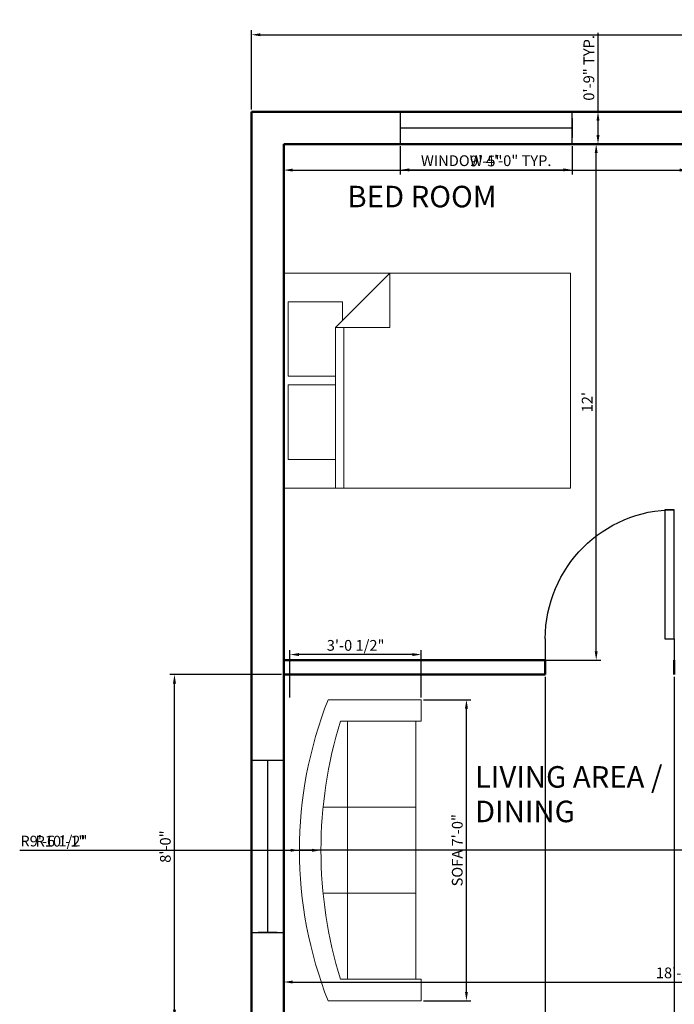
# Model space of a CAD drawing. Units: inches. Extents: x 1767 to 2185, y 3382 to 3854.
# Tile 2 of 4: x 1767 to 1950, y 3577 to 3852. Entities that reach past the tile are written whole.
import ezdxf

# ---------------------------------------------------------------- set-up
doc = ezdxf.new("R2010")
doc.units = ezdxf.units.IN
for name, color, linetype, lineweight in [('A-ANNO-DIMS', 2, 'Continuous', 18), ('A-AREA-IDEN', 7, 'Continuous', 25), ('A-DOOR', 3, 'Continuous', 25), ('A-FURN', 8, 'Continuous', 18), ('A-GLAZ', 4, 'Continuous', 25), ('A-WALL', 7, 'Continuous', 50)]:
    doc.layers.add(name, color=color, linetype=linetype, lineweight=lineweight)
doc.styles.get("Standard").update_dxf_attribs({"font": 'arial.ttf'})
doc.dimstyles.new('ISO-25', dxfattribs={"dimtxt": 3, "dimasz": 2.5, "dimexe": 1.25, "dimexo": 0.625, "dimtad": 1, "dimdec": 0, "dimlunit": 3, "dimtxsty": 'Standard', "dimcen": 2.5, "dimadec": 0, "dimazin": 0, "dimtfac": 1, "dimtdec": 0, "dimtmove": 0, "dimatfit": 3, "dimfxl": 1, "dimarcsym": 0})

# ---------------------------------------------------------------- blocks, each defined once
blk = doc.blocks.new('*U2')
for p, q in [((0, 0), (0, -100)), ((600, 0), (600, -100))]:
    blk.add_line(p, q)
blk.add_lwpolyline([(0, 0), (0, 600), (43.75, 600), (43.75, 0)], close=True)
blk.add_arc((0, 0), 600, 0, 90)
blk = doc.blocks.new('*U4')
for p, q in [((0, 100), (0, 0)), ((900, 100), (900, 0)), ((0, 50), (900, 50))]:
    blk.add_line(p, q)
blk = doc.blocks.new('Bed - Queen')
for p, q in [((0, -80.00003), (0, 0)), ((0, 0), (59.99999, 0)), ((59.99999, 0), (59.99999, -80.00003)), ((7.99999, -1.2), (28.79998, -1.2)), ((7.99999, -14.4), (7.99999, -1.2)), ((28.79998, -1.2), (28.79998, -14.4)), ((31.19999, -1.2), (51.99999, -1.2)), ((31.19999, -14.4), (31.19999, -1.2)), ((51.99999, -1.2), (51.99999, -16.4)), ((0, -14.4), (44.8, -14.4)), ((59.99999, -29.6), (44.8, -14.4)), ((44.8, -14.4), (44.8, -29.6)), ((51.99999, -16.4), (46.79936, -16.4)), ((44.8, -16.8), (0, -16.8)), ((44.8, -29.6), (59.99999, -29.6)), ((59.99999, -80.00003), (0, -80.00003))]:
    blk.add_line(p, q)
blk = doc.blocks.new('Sofa - Roundback 7 ft.')
for p, q in [((-12.00002, -32.4421), (-12.00003, -6.5971)), ((11.99997, -32.4421), (11.99998, -6.5971)), ((-36.000027, -34), (-36.000027, -11.4696)), ((-35.999844, -13.3819), (35.9998, -13.3819)), ((35.99998, -34), (35.99998, -11.4696)), ((-36.000027, -32.4421), (35.99998, -32.4421))]:
    blk.add_line(p, q)
for points in [[(-36.000027, -34), (-42.000027, -34), (-42.000027, -8)], [(41.99998, -8), (41.99998, -34), (35.99998, -34)]]:
    blk.add_lwpolyline(points)
for centre, radius, start, end in [((0, -114.25), 114.25, 68.43141, 111.5686), ((-0.00001, -127.1968), 121.1968, 72.72033, 107.2797)]:
    blk.add_arc(centre, radius, start, end)
blk = doc.blocks.new('*D10')
at = {"layer": 'A-ANNO-DIMS', "color": 0, "lineweight": -2, "transparency": 16777216}
for p, q in [((1841.16, 3816.53), (1841.16, 3808.64)), ((1954.16, 3816.53), (1954.16, 3808.64)), ((1843.66, 3809.89), (1951.66, 3809.89))]:
    blk.add_line(p, q, dxfattribs=at)
at = {"layer": 'A-ANNO-DIMS', "color": 0, "transparency": 16777216}
for points in [[(1843.66, 3810.31), (1843.66, 3809.48), (1841.16, 3809.89)], [(1951.66, 3810.31), (1951.66, 3809.48), (1954.16, 3809.89)]]:
    blk.add_solid(points, dxfattribs=at)
at = {"layer": 'Defpoints', "color": 0, "transparency": 16777216}
for p in [(1841.16, 3817.15), (1954.16, 3817.15), (1954.16, 3809.89)]:
    blk.add_point(p, dxfattribs=at)
at = {"layer": 'A-ANNO-DIMS', "color": 0, "transparency": 16777216, "insert": (1897.66, 3812.05), "char_height": 3, "attachment_point": 5}
blk.add_mtext('9\'-5"', dxfattribs=at)
blk = doc.blocks.new('*D11')
at = {"layer": 'A-ANNO-DIMS', "color": 0, "lineweight": -2, "transparency": 16777216}
for p, q in [((1841.78, 3817.15), (1929.61, 3817.15)), ((1928.36, 3675.65), (1928.36, 3814.65)), ((1841.78, 3673.15), (1929.61, 3673.15))]:
    blk.add_line(p, q, dxfattribs=at)
at = {"layer": 'A-ANNO-DIMS', "color": 0, "transparency": 16777216}
for points in [[(1927.94, 3814.65), (1928.77, 3814.65), (1928.36, 3817.15)], [(1927.94, 3675.65), (1928.77, 3675.65), (1928.36, 3673.15)]]:
    blk.add_solid(points, dxfattribs=at)
at = {"layer": 'Defpoints', "color": 0, "transparency": 16777216}
for p in [(1841.16, 3817.15), (1928.36, 3817.15), (1841.16, 3673.15)]:
    blk.add_point(p, dxfattribs=at)
at = {"layer": 'A-ANNO-DIMS', "color": 0, "transparency": 16777216, "insert": (1926.23, 3745.15), "char_height": 3, "attachment_point": 5, "rotation": 90}
blk.add_mtext("12'", dxfattribs=at)
blk = doc.blocks.new('*D17')
at = {"layer": 'A-ANNO-DIMS', "color": 0, "lineweight": -2, "transparency": 16777216}
for p, q in [((1841.16, 3668.53), (1841.16, 3582.12)), ((2060.16, 3668.53), (2060.16, 3582.12)), ((1843.66, 3583.37), (2057.66, 3583.37))]:
    blk.add_line(p, q, dxfattribs=at)
at = {"layer": 'A-ANNO-DIMS', "color": 0, "transparency": 16777216}
for points in [[(1843.66, 3583.79), (1843.66, 3582.96), (1841.16, 3583.37)], [(2057.66, 3583.79), (2057.66, 3582.96), (2060.16, 3583.37)]]:
    blk.add_solid(points, dxfattribs=at)
at = {"layer": 'Defpoints', "color": 0, "transparency": 16777216}
for p in [(1841.16, 3669.15), (2060.16, 3669.15), (2060.16, 3583.37)]:
    blk.add_point(p, dxfattribs=at)
at = {"layer": 'A-ANNO-DIMS', "color": 0, "transparency": 16777216, "insert": (1950.66, 3585.53), "char_height": 3, "attachment_point": 5}
blk.add_mtext('18\'-3"', dxfattribs=at)
blk = doc.blocks.new('WIN-OPENING-48IN-WALL-9IN')
for p, q in [((48, 9), (0, 9)), ((0, 9), (0, 0)), ((48, 0), (48, 9))]:
    blk.add_line(p, q)
blk = doc.blocks.new('*D27')
at = {"layer": 'A-ANNO-DIMS', "color": 0, "lineweight": -2, "transparency": 16777216}
for p, q in [((1873.66, 3816.53), (1873.66, 3808.7)), ((1921.66, 3816.53), (1921.66, 3808.7)), ((1876.16, 3809.95), (1919.16, 3809.95))]:
    blk.add_line(p, q, dxfattribs=at)
at = {"layer": 'A-ANNO-DIMS', "color": 0, "transparency": 16777216}
for points in [[(1876.16, 3810.37), (1876.16, 3809.53), (1873.66, 3809.95)], [(1919.16, 3810.37), (1919.16, 3809.53), (1921.66, 3809.95)]]:
    blk.add_solid(points, dxfattribs=at)
at = {"layer": 'Defpoints', "color": 0, "transparency": 16777216}
for p in [(1873.66, 3817.15), (1921.66, 3817.15), (1921.66, 3809.95)]:
    blk.add_point(p, dxfattribs=at)
at = {"layer": 'A-ANNO-DIMS', "color": 0, "transparency": 16777216, "insert": (1897.66, 3812.13), "char_height": 3, "attachment_point": 5}
blk.add_mtext('WINDOW 4\'-0" TYP.', dxfattribs=at)
blk = doc.blocks.new('*D28')
at = {"layer": 'A-ANNO-DIMS', "color": 0, "lineweight": -2, "transparency": 16777216}
for p, q in [((1928.86, 3826.15), (1928.86, 3848.19)), ((1922.28, 3826.15), (1930.11, 3826.15)), ((1928.86, 3819.65), (1928.86, 3823.65)), ((1922.28, 3817.15), (1930.11, 3817.15))]:
    blk.add_line(p, q, dxfattribs=at)
at = {"layer": 'A-ANNO-DIMS', "color": 0, "transparency": 16777216}
for points in [[(1928.44, 3823.65), (1929.28, 3823.65), (1928.86, 3826.15)], [(1928.44, 3819.65), (1929.28, 3819.65), (1928.86, 3817.15)]]:
    blk.add_solid(points, dxfattribs=at)
at = {"layer": 'Defpoints', "color": 0, "transparency": 16777216}
for p in [(1921.66, 3826.15), (1928.86, 3826.15), (1921.66, 3817.15)]:
    blk.add_point(p, dxfattribs=at)
at = {"layer": 'A-ANNO-DIMS', "color": 0, "transparency": 16777216, "insert": (1926.7, 3838.42), "char_height": 3, "attachment_point": 5, "rotation": 90}
blk.add_mtext('0\'-9" TYP.', dxfattribs=at)
blk = doc.blocks.new('*D37')
at = {"layer": 'A-ANNO-DIMS', "color": 0, "lineweight": -2, "transparency": 16777216}
for p, q in [((1880.17, 3662.13), (1893.39, 3662.13)), ((1892.14, 3580.63), (1892.14, 3659.63)), ((1880.17, 3578.13), (1893.39, 3578.13))]:
    blk.add_line(p, q, dxfattribs=at)
at = {"layer": 'A-ANNO-DIMS', "color": 0, "transparency": 16777216}
for points in [[(1891.73, 3659.63), (1892.56, 3659.63), (1892.14, 3662.13)], [(1891.73, 3580.63), (1892.56, 3580.63), (1892.14, 3578.13)]]:
    blk.add_solid(points, dxfattribs=at)
at = {"layer": 'Defpoints', "color": 0, "transparency": 16777216}
for p in [(1879.54, 3662.13), (1892.14, 3662.13), (1879.54, 3578.13)]:
    blk.add_point(p, dxfattribs=at)
at = {"layer": 'A-ANNO-DIMS', "color": 0, "transparency": 16777216, "insert": (1889.97, 3620.13), "char_height": 3, "attachment_point": 5, "rotation": 90}
blk.add_mtext('SOFA 7\'-0"', dxfattribs=at)
blk = doc.blocks.new('*D38')
at = {"layer": 'A-ANNO-DIMS', "color": 0, "lineweight": -2, "transparency": 16777216}
for p, q in [((1842.88, 3662.75), (1842.88, 3675.98)), ((1879.54, 3662.75), (1879.54, 3675.98)), ((1877.04, 3674.73), (1845.38, 3674.73))]:
    blk.add_line(p, q, dxfattribs=at)
at = {"layer": 'A-ANNO-DIMS', "color": 0, "transparency": 16777216}
for points in [[(1845.38, 3675.14), (1845.38, 3674.31), (1842.88, 3674.73)], [(1877.04, 3675.14), (1877.04, 3674.31), (1879.54, 3674.73)]]:
    blk.add_solid(points, dxfattribs=at)
at = {"layer": 'Defpoints', "color": 0, "transparency": 16777216}
for p in [(1842.88, 3674.73), (1842.88, 3662.13), (1879.54, 3662.13)]:
    blk.add_point(p, dxfattribs=at)
at = {"layer": 'A-ANNO-DIMS', "color": 0, "transparency": 16777216, "insert": (1861.21, 3676.9), "char_height": 3, "attachment_point": 5}
blk.add_mtext('3\'-0 1/2"', dxfattribs=at)
blk = doc.blocks.new('*D39')
at = {"layer": 'A-ANNO-DIMS', "color": 0, "lineweight": -2, "transparency": 16777216}
for p, q in [((1832.16, 3826.78), (1832.16, 3848.91)), ((2144.16, 3826.78), (2144.16, 3848.91)), ((1834.66, 3847.66), (2141.66, 3847.66))]:
    blk.add_line(p, q, dxfattribs=at)
at = {"layer": 'A-ANNO-DIMS', "color": 0, "transparency": 16777216}
for points in [[(1834.66, 3848.07), (1834.66, 3847.24), (1832.16, 3847.66)], [(2141.66, 3848.07), (2141.66, 3847.24), (2144.16, 3847.66)]]:
    blk.add_solid(points, dxfattribs=at)
at = {"layer": 'Defpoints', "color": 0, "transparency": 16777216}
for p in [(2144.16, 3847.66), (1832.16, 3826.15), (2144.16, 3826.15)]:
    blk.add_point(p, dxfattribs=at)
at = {"layer": 'A-ANNO-DIMS', "color": 0, "transparency": 16777216, "insert": (1988.16, 3849.81), "char_height": 3, "attachment_point": 5}
blk.add_mtext('26\'-0"', dxfattribs=at)
blk = doc.blocks.new('*D41')
at = {"layer": 'A-ANNO-DIMS', "color": 0, "lineweight": -2, "transparency": 16777216}
for p, q in [((1840.53, 3669.15), (1809.4, 3669.15)), ((1810.65, 3575.65), (1810.65, 3666.65)), ((1831.53, 3573.15), (1809.4, 3573.15))]:
    blk.add_line(p, q, dxfattribs=at)
at = {"layer": 'A-ANNO-DIMS', "color": 0, "transparency": 16777216}
for points in [[(1810.24, 3666.65), (1811.07, 3666.65), (1810.65, 3669.15)], [(1810.24, 3575.65), (1811.07, 3575.65), (1810.65, 3573.15)]]:
    blk.add_solid(points, dxfattribs=at)
at = {"layer": 'Defpoints', "color": 0, "transparency": 16777216}
for p in [(1810.65, 3669.15), (1841.16, 3669.15), (1832.16, 3573.15)]:
    blk.add_point(p, dxfattribs=at)
at = {"layer": 'A-ANNO-DIMS', "color": 0, "transparency": 16777216, "insert": (1808.5, 3621.15), "char_height": 3, "attachment_point": 5, "rotation": 90}
blk.add_mtext('8\'-0"', dxfattribs=at)
blk = doc.blocks.new('*D42')
at = {"layer": 'A-ANNO-DIMS', "color": 0, "lineweight": -2, "transparency": 16777216}
for p, q in [((1914.16, 3668.53), (1914.16, 3383.4)), ((1950.16, 3668.53), (1950.16, 3383.4)), ((1916.66, 3384.65), (1947.66, 3384.65))]:
    blk.add_line(p, q, dxfattribs=at)
at = {"layer": 'A-ANNO-DIMS', "color": 0, "transparency": 16777216}
for points in [[(1916.66, 3385.06), (1916.66, 3384.23), (1914.16, 3384.65)], [(1947.66, 3385.06), (1947.66, 3384.23), (1950.16, 3384.65)]]:
    blk.add_solid(points, dxfattribs=at)
at = {"layer": 'Defpoints', "color": 0, "transparency": 16777216}
for p in [(1914.16, 3669.15), (1950.16, 3669.15), (1950.16, 3384.65)]:
    blk.add_point(p, dxfattribs=at)
at = {"layer": 'A-ANNO-DIMS', "color": 0, "transparency": 16777216, "insert": (1932.16, 3386.8), "char_height": 3, "attachment_point": 5}
blk.add_mtext('3\'-0"', dxfattribs=at)
blk = doc.blocks.new('*D51')
at = {"layer": 'A-ANNO-DIMS', "color": 0, "lineweight": -2, "transparency": 16777216}
for p, q in [((1771.61, 3620.13), (1849.04, 3620.13)), ((1972.74, 3620.13), (1851.54, 3620.13))]:
    blk.add_line(p, q, dxfattribs=at)
at = {"layer": 'A-ANNO-DIMS', "color": 0, "transparency": 16777216}
blk.add_solid([(1849.04, 3620.54), (1849.04, 3619.71), (1851.54, 3620.13)], dxfattribs=at)
at = {"layer": 'Defpoints', "color": 0, "transparency": 16777216}
for p in [(1851.54, 3620.13), (1972.74, 3620.13)]:
    blk.add_point(p, dxfattribs=at)
at = {"layer": 'A-ANNO-DIMS', "color": 0, "transparency": 16777216, "insert": (1778.83, 3622.28), "char_height": 3, "attachment_point": 5, "rotation": 359.9999}
blk.add_mtext('R10\'-1"', dxfattribs=at)
blk = doc.blocks.new('*D52')
at = {"layer": 'A-ANNO-DIMS', "color": 0, "lineweight": -2, "transparency": 16777216}
for p, q in [((1767.45, 3620.13), (1843.04, 3620.13)), ((1959.79, 3620.13), (1845.54, 3620.13))]:
    blk.add_line(p, q, dxfattribs=at)
at = {"layer": 'A-ANNO-DIMS', "color": 0, "transparency": 16777216}
blk.add_solid([(1843.04, 3620.54), (1843.04, 3619.71), (1845.54, 3620.13)], dxfattribs=at)
at = {"layer": 'Defpoints', "color": 0, "transparency": 16777216}
for p in [(1845.54, 3620.13), (1959.79, 3620.13)]:
    blk.add_point(p, dxfattribs=at)
at = {"layer": 'A-ANNO-DIMS', "color": 0, "transparency": 16777216, "insert": (1776.99, 3622.3), "char_height": 3, "attachment_point": 5, "rotation": 359.9999}
blk.add_mtext('R9\'-6 1/2"', dxfattribs=at)

msp = doc.modelspace()

# ---------------------------------------------------------------- linework, layer by layer
at = {"layer": 'A-WALL'}
for p, q in [((1832.16, 3826.15), (2144.16, 3826.15)), ((1832.16, 3406.15), (1832.16, 3826.15)), ((1841.16, 3415.15), (1841.16, 3817.15)), ((1841.16, 3817.15), (2135.16, 3817.15)), ((1841.16, 3673.15), (1914.16, 3673.15)), ((1914.16, 3673.15), (1914.16, 3669.15)), ((1950.16, 3669.15), (1950.16, 3673.15)), ((1841.16, 3669.15), (1914.16, 3669.15))]:
    msp.add_line(p, q, dxfattribs=at)

# ---------------------------------------------------------------- block references
at = {"layer": 'A-DOOR', "xscale": -0.0599999999999998, "yscale": 0.0599999999999998, "zscale": 0.0599999999999998}
msp.add_blockref('*U2', (1950.16, 3679.15), dxfattribs=at)
at = {"layer": 'A-FURN', "rotation": 90}
for name, p in [('Bed - Queen', (1841.16, 3721.16)), ('Sofa - Roundback 7 ft.', (1845.54, 3620.13))]:
    msp.add_blockref(name, p, dxfattribs=at)
at = {"layer": 'A-GLAZ'}
msp.add_blockref('WIN-OPENING-48IN-WALL-9IN', (1873.66, 3817.15), dxfattribs=at)
at = {"layer": 'A-GLAZ', "xscale": 0.0533333333333335, "yscale": 0.0533333333333335, "zscale": 0.0533333333333335}
msp.add_blockref('*U4', (1873.66, 3818.98), dxfattribs=at)
at = {"layer": 'A-GLAZ', "rotation": 90.00000000000126}
msp.add_blockref('WIN-OPENING-48IN-WALL-9IN', (1841.16, 3597.15), dxfattribs=at)
at = {"layer": 'A-GLAZ', "xscale": 0.0533333333333335, "yscale": 0.0533333333333335, "zscale": 0.0533333333333335, "rotation": 270}
msp.add_blockref('*U4', (1833.99, 3645.15), dxfattribs=at)

# ---------------------------------------------------------------- texts
at = {"layer": 'A-AREA-IDEN'}
for s, p in [('BED ROOM', (1858.91, 3799.51)), ('LIVING AREA /', (1894.5, 3637.6)), ('DINING', (1894.5, 3627.96))]:
    msp.add_text(s, height=6, dxfattribs=at).set_placement(p)

# ---------------------------------------------------------------- dimensions: what is measured, and where the dimension line sits
at = {"layer": 'A-ANNO-DIMS'}
for base, p1, p2, override, picture, middle in [((2144.16, 3847.66), (1832.16, 3826.15), (2144.16, 3826.15), {"dimdec": 1, "dimlfac": 1, "dimrnd": 0, "dimzin": 1, "dimdsep": 46, "dimlunit": 4, "dimfrac": 2}, '*D39', (1988.16, 3849.81)), ((1954.16, 3809.89), (1841.16, 3817.15), (1954.16, 3817.15), {"dimclrd": 0, "dimclre": 0, "dimclrt": 0}, '*D10', (1897.66, 3812.05)), ((2060.16, 3583.37), (1841.16, 3669.15), (2060.16, 3669.15), {"dimclrd": 0, "dimclre": 0, "dimclrt": 0}, '*D17', (1950.66, 3585.53)), ((1950.16, 3384.65), (1914.16, 3669.15), (1950.16, 3669.15), {"dimdec": 1, "dimlfac": 1, "dimrnd": 0, "dimzin": 1, "dimdsep": 46, "dimlunit": 4, "dimfrac": 2}, '*D42', (1932.16, 3386.8))]:
    dim = msp.add_linear_dim(base=base, p1=p1, p2=p2, dimstyle='ISO-25', override=override, dxfattribs=at)
    dim.commit()
    dim.dimension.update_dxf_attribs({"geometry": picture, "text_midpoint": middle})
for base, p1, p2, text, picture, middle in [((1928.86, 3826.15), (1921.66, 3817.15), (1921.66, 3826.15), '<> TYP.', '*D28', (1926.7, 3838.42)), ((1892.14, 3662.13), (1879.54, 3578.13), (1879.54, 3662.13), 'SOFA <>', '*D37', (1889.97, 3620.13))]:
    dim = msp.add_linear_dim(base=base, p1=p1, p2=p2, angle=90, text=text, dimstyle='ISO-25', override={"dimdec": 1, "dimlfac": 1, "dimrnd": 0, "dimzin": 1, "dimdsep": 46, "dimlunit": 4, "dimfrac": 2}, dxfattribs=at)
    dim.commit()
    dim.dimension.update_dxf_attribs({"geometry": picture, "text_midpoint": middle})
dim = msp.add_linear_dim(base=(1921.66, 3809.95), p1=(1873.66, 3817.15), p2=(1921.66, 3817.15), text='WINDOW <> TYP.', dimstyle='ISO-25', override={"dimdec": 1, "dimlfac": 1, "dimrnd": 0, "dimzin": 1, "dimdsep": 46, "dimlunit": 4, "dimfrac": 2}, dxfattribs=at)
dim.commit()
dim.dimension.update_dxf_attribs({"geometry": '*D27', "text_midpoint": (1897.66, 3812.13)})
for base, p1, p2, angle, override, picture, middle in [((1928.36, 3817.15), (1841.16, 3673.15), (1841.16, 3817.15), 90, {"dimclrd": 0, "dimclre": 0, "dimclrt": 0}, '*D11', (1926.23, 3745.15)), ((1842.88, 3674.73), (1879.54, 3662.13), (1842.88, 3662.13), 180, {"dimdec": 1, "dimlfac": 1, "dimrnd": 0, "dimzin": 1, "dimdsep": 46, "dimlunit": 4, "dimfrac": 2}, '*D38', (1861.21, 3676.9)), ((1810.65, 3669.15), (1832.16, 3573.15), (1841.16, 3669.15), 90, {"dimdec": 1, "dimlfac": 1, "dimrnd": 0, "dimzin": 1, "dimdsep": 46, "dimlunit": 4, "dimfrac": 2}, '*D41', (1808.5, 3621.15))]:
    dim = msp.add_linear_dim(base=base, p1=p1, p2=p2, angle=angle, dimstyle='ISO-25', override=override, dxfattribs=at)
    dim.commit()
    dim.dimension.update_dxf_attribs({"geometry": picture, "text_midpoint": middle})
for center, mpoint, picture, middle in [((1959.793426, 3620.126703), (1845.543426, 3620.127), '*D52', (1776.993426, 3620.1271782)), ((1972.74, 3620.13), (1851.54, 3620.13), '*D51', (1778.83, 3620.13))]:
    dim = msp.add_radius_dim(center=center, mpoint=mpoint, dimstyle='ISO-25', override={"dimdec": 1, "dimlfac": 1, "dimrnd": 0, "dimzin": 1, "dimdsep": 46, "dimlunit": 4, "dimfrac": 2}, dxfattribs=at)
    dim.commit()
    dim.dimension.update_dxf_attribs({"geometry": picture, "text_midpoint": middle, "dimtype": 164})

doc.saveas('drawing.dxf')
